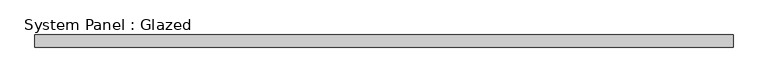
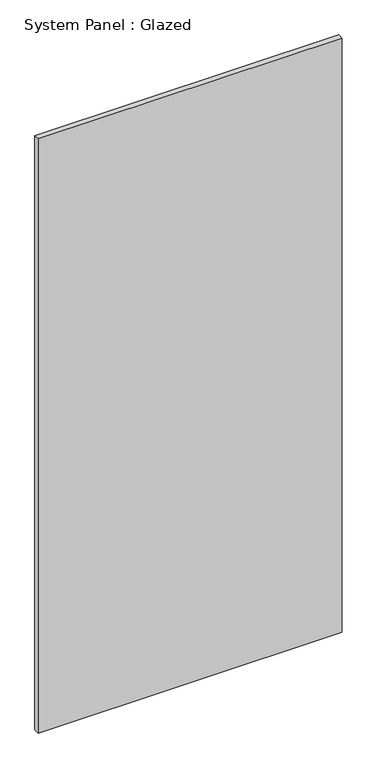
"""IFC4 building model written with IfcOpenShell, lengths in millimetres: plate geometry, System Panel : Glazed."""

from ifc_helpers import new_model, si_unit, origin, origin_with_axes, place, context, project, spatial, polyline, outline, extrude, source, transform, mapped, element, save


def system_panel_glazed_395abe7e(model_context):
    return source(origin(), model_context, "Body", "SweptSolid", [
        extrude(outline(polyline([(707.7208312, 19.05), (-707.7208312, 19.05), (-707.7208312, 44.45), (707.7208312, 44.45), (707.7208312, 19.05)])), origin_with_axes(), (0.0, 0.0, 1.0), 2921.0),
    ])


if __name__ == "__main__":
    model = new_model("IFC4")
    model_context = context("Model", 3, world=origin())
    ifc_project = project(units=[si_unit("LENGTHUNIT", "METRE", prefix="MILLI")], contexts=[model_context])
    site = spatial("IfcSite", under=ifc_project)
    building = spatial("IfcBuilding", under=site)
    placement = place(None, origin())
    system_panel_glazed_shape = system_panel_glazed_395abe7e(model_context)
    element("IfcPlate", 1, ObjectType="System Panel : Glazed", at=placement, inside=building, context=model_context, shape_type="MappedRepresentation", body=[
        mapped(system_panel_glazed_shape, transform((0.0, 0.0, 0.0), x_axis=(1.0, 0.0, 0.0), y_axis=(0.0, 1.0, 0.0), z_axis=(0.0, 0.0, 1.0))),
    ])
    save(model, "model.ifc")

# Revit data of these elements
# Type "System Panel : Glazed"
#   Construction Type Id = "GSP4R"
#   Analytic Construction = "1/8 in Pilkington single glazing"
#   Visual Light Transmittance = 0.9
#   Solar Heat Gain Coefficient = 0.86
#   Heat Transfer Coefficient (U) = 1.18115 BTU/(h·ft²·°F)
# Element 1 (IfcPlate, "System Panel : Glazed")
#   Materials on its faces: "Glass"
# Materials
#   "Glass": class "Glass", colour RGB 0 128 192, transparency 0.75, Description = "Soda Lime Glass", Cost = 0
